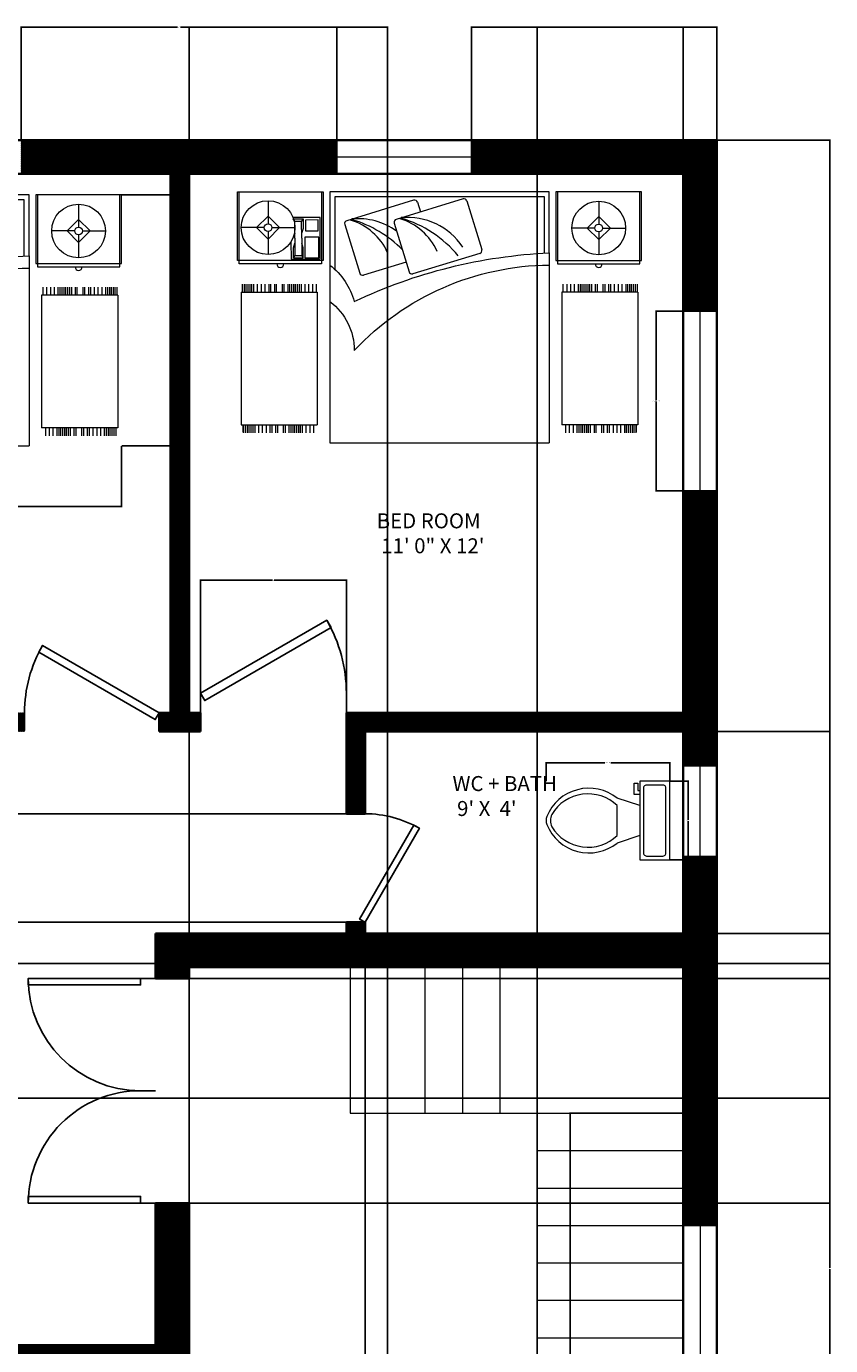
# Model space of a CAD drawing. Units: inches. Extents: x -24 to 516, y -23 to 640.
# Tile 5 of 5: x 302 to 516, y 288 to 640. Entities that reach past the tile are written whole.
import ezdxf

# ---------------------------------------------------------------- set-up
doc = ezdxf.new("R2010")
doc.units = ezdxf.units.IN
doc.header["$MEASUREMENT"] = 0
for name, color, linetype, lineweight in [('A-ANNO-DIMS', 2, 'Continuous', 18), ('A-AREA-IDEN', 7, 'Continuous', 18), ('A-FLOR-STRS', 7, 'Continuous', 18), ('A-WALL', 7, 'Continuous', 35), ('bathroom', 90, 'Continuous', 18), ('bedroom', 120, 'Continuous', 18), ('doors', 40, 'Continuous', 25), ('window', 30, 'Continuous', 18)]:
    doc.layers.add(name, color=color, linetype=linetype, lineweight=lineweight)
doc.layers.add('A-WALL-PATT', color=198, linetype='Continuous', lineweight=13, true_color=0x2e0f2e)
doc.styles.get("Standard").update_dxf_attribs({"font": 'arial.ttf'})
doc.dimstyles.get("Standard").update_dxf_attribs({"dimtxt": 0.18, "dimasz": 0.18, "dimexe": 0.18, "dimexo": 0.0625, "dimgap": 0.09, "dimtad": 0, "dimtih": 1, "dimtoh": 1, "dimdec": 4, "dimzin": 0, "dimdsep": 46, "dimtxsty": 'Standard', "dimcen": 0.09, "dimadec": 0, "dimazin": 0, "dimtfac": 1, "dimtdec": 4, "dimtofl": 0, "dimtmove": 0, "dimatfit": 3, "dimfxl": 1, "dimtolj": 1, "dimtzin": 0, "dimarcsym": 0})
pattern_1 = [(45, (-12045.43418, -42625.98622), (-0.08838834765, 0.08838834765), [])]

# ---------------------------------------------------------------- blocks, each defined once
blk = doc.blocks.new('*U6')
for p, q in [((0, 0), (0, -100)), ((750, 0), (750, -100))]:
    blk.add_line(p, q)
blk.add_lwpolyline([(0, 0), (649.5, 375), (671.4, 337.1), (21.9, -37.9)], close=True)
blk.add_arc((0, 0), 750, 0, 30)
blk = doc.blocks.new('*U7')
for p, q in [((0, 0), (0, 100)), ((750, 0), (750, 100))]:
    blk.add_line(p, q)
blk.add_lwpolyline([(0, 0), (649.5, -375), (671.4, -337.1), (21.9, 37.9)], close=True)
blk.add_arc((0, 0), 750, 330, 0)
blk = doc.blocks.new('*U9')
for p, q in [((0, 0), (0, -100)), ((750, 0), (750, -100))]:
    blk.add_line(p, q)
blk.add_lwpolyline([(0, 0), (0, 750), (43.75, 750), (43.75, 0)], close=True)
blk.add_arc((0, 0), 750, 0, 90)
blk = doc.blocks.new('3')
for p, q in [((185.866, 224.677), (185.866, 225.236)), ((185.866, 225.236), (186.566, 225.236)), ((185.88, 224.649), (185.88, 225.236)), ((186.552, 225.236), (186.552, 224.649)), ((186.566, 225.236), (186.566, 224.677)), ((186.62, 225.236), (186.62, 224.64)), ((188.409, 225.236), (186.62, 225.236)), ((188.409, 224.739), (188.409, 225.236)), ((188.463, 225.236), (188.463, 224.677)), ((189.162, 225.236), (188.463, 225.236)), ((188.477, 225.236), (188.477, 224.649)), ((189.148, 224.649), (189.148, 225.236)), ((189.162, 224.677), (189.162, 225.236)), ((186.116, 225.164), (186.116, 224.976)), ((187.303, 225.168), (186.758, 225.001)), ((187.706, 225.179), (187.161, 225.012)), ((187.334, 225.152), (187.359, 225.073)), ((187.737, 225.163), (187.858, 224.766)), ((188.812, 225.162), (188.812, 224.974)), ((186.022, 224.945), (186.116, 225.039)), ((186.116, 225.039), (186.21, 224.945)), ((186.54, 225.027), (186.319, 225.027)), ((186.321, 225.017), (186.401, 225.017)), ((186.401, 225.017), (186.389, 224.997)), ((186.401, 225.017), (186.401, 224.938)), ((186.541, 224.69), (186.54, 225.027)), ((188.812, 225.036), (188.718, 224.942)), ((188.907, 224.942), (188.812, 225.036)), ((186.084, 224.945), (185.896, 224.945)), ((186.116, 224.851), (186.022, 224.945)), ((186.21, 224.945), (186.116, 224.851)), ((186.116, 224.914), (186.116, 224.726)), ((186.147, 224.945), (186.335, 224.945)), ((186.333, 224.997), (186.321, 225.017)), ((186.334, 224.858), (186.333, 224.997)), ((186.333, 224.997), (186.389, 224.997)), ((186.39, 224.858), (186.389, 224.997)), ((186.401, 224.938), (186.389, 224.898)), ((186.742, 224.97), (186.863, 224.573)), ((187.144, 224.981), (187.266, 224.584)), ((188.781, 224.942), (188.593, 224.942)), ((188.718, 224.942), (188.812, 224.848)), ((188.812, 224.848), (188.907, 224.942)), ((188.812, 224.911), (188.812, 224.723)), ((188.844, 224.942), (189.032, 224.942)), ((186.302, 224.83), (186.303, 224.689)), ((186.322, 224.779), (186.334, 224.818)), ((186.331, 224.905), (186.334, 224.898)), ((186.334, 224.858), (186.334, 224.719)), ((186.39, 224.858), (186.39, 224.719)), ((186.402, 224.779), (186.39, 224.819)), ((186.323, 224.699), (186.322, 224.779)), ((186.334, 224.719), (186.323, 224.699)), ((186.323, 224.699), (186.402, 224.7)), ((186.334, 224.719), (186.39, 224.719)), ((186.402, 224.7), (186.39, 224.719)), ((186.402, 224.7), (186.402, 224.779)), ((187.842, 224.735), (187.297, 224.568)), ((188.409, 224.739), (188.409, 223.191)), ((186.566, 224.677), (185.866, 224.677)), ((186.552, 224.649), (185.88, 224.649)), ((186.303, 224.689), (186.541, 224.69)), ((186.62, 224.64), (186.62, 223.191)), ((187.242, 224.663), (186.894, 224.557)), ((188.463, 224.677), (189.162, 224.677)), ((188.477, 224.649), (189.148, 224.649)), ((185.904, 224.485, -0.909), (185.904, 224.42, -0.909)), ((185.92, 224.485, -0.909), (185.92, 224.42, -0.909)), ((185.92, 224.485, -0.909), (185.92, 224.42, -0.909)), ((185.935, 224.485, -0.909), (185.935, 224.42, -0.909)), ((185.951, 224.485, -0.909), (185.951, 224.42, -0.909)), ((185.966, 224.485, -0.909), (185.966, 224.42, -0.909)), ((185.982, 224.485, -0.909), (185.982, 224.42, -0.909)), ((185.997, 224.485, -0.909), (185.997, 224.42, -0.909)), ((186.028, 224.485, -0.909), (186.028, 224.42, -0.909)), ((186.059, 224.485, -0.909), (186.059, 224.42, -0.909)), ((186.09, 224.485, -0.909), (186.09, 224.42, -0.909)), ((186.09, 224.485, -0.909), (186.09, 224.42, -0.909)), ((186.121, 224.485, -0.909), (186.121, 224.42, -0.909)), ((186.137, 224.485, -0.909), (186.137, 224.42, -0.909)), ((186.168, 224.485, -0.909), (186.168, 224.42, -0.909)), ((186.183, 224.485, -0.909), (186.183, 224.42, -0.909)), ((186.23, 224.485, -0.909), (186.23, 224.42, -0.909)), ((186.245, 224.485, -0.909), (186.245, 224.42, -0.909)), ((186.276, 224.485, -0.909), (186.276, 224.42, -0.909)), ((186.292, 224.485, -0.909), (186.292, 224.42, -0.909)), ((186.307, 224.485, -0.909), (186.307, 224.42, -0.909)), ((186.323, 224.485, -0.909), (186.323, 224.42, -0.909)), ((186.338, 224.485, -0.909), (186.338, 224.42, -0.909)), ((186.354, 224.485, -0.909), (186.354, 224.42, -0.909)), ((186.369, 224.485, -0.909), (186.369, 224.42, -0.909)), ((186.385, 224.485, -0.909), (186.385, 224.42, -0.909)), ((186.416, 224.485, -0.909), (186.416, 224.42, -0.909)), ((186.447, 224.485, -0.909), (186.447, 224.42, -0.909)), ((186.478, 224.485, -0.909), (186.478, 224.42, -0.909)), ((186.509, 224.485, -0.909), (186.509, 224.42, -0.909)), ((188.52, 224.485, -0.909), (188.52, 224.42, -0.909)), ((188.551, 224.485, -0.909), (188.551, 224.42, -0.909)), ((188.582, 224.485, -0.909), (188.582, 224.42, -0.909)), ((188.613, 224.485, -0.909), (188.613, 224.42, -0.909)), ((188.644, 224.485, -0.909), (188.644, 224.42, -0.909)), ((188.66, 224.485, -0.909), (188.66, 224.42, -0.909)), ((188.675, 224.485, -0.909), (188.675, 224.42, -0.909)), ((188.691, 224.485, -0.909), (188.691, 224.42, -0.909)), ((188.706, 224.485, -0.909), (188.706, 224.42, -0.909)), ((188.722, 224.485, -0.909), (188.722, 224.42, -0.909)), ((188.737, 224.485, -0.909), (188.737, 224.42, -0.909)), ((188.753, 224.485, -0.909), (188.753, 224.42, -0.909)), ((188.784, 224.485, -0.909), (188.784, 224.42, -0.909)), ((188.799, 224.485, -0.909), (188.799, 224.42, -0.909)), ((188.846, 224.485, -0.909), (188.846, 224.42, -0.909)), ((188.861, 224.485, -0.909), (188.861, 224.42, -0.909)), ((188.892, 224.485, -0.909), (188.892, 224.42, -0.909)), ((188.908, 224.485, -0.909), (188.908, 224.42, -0.909)), ((188.939, 224.485, -0.909), (188.939, 224.42, -0.909)), ((188.939, 224.485, -0.909), (188.939, 224.42, -0.909)), ((188.97, 224.485, -0.909), (188.97, 224.42, -0.909)), ((189.001, 224.485, -0.909), (189.001, 224.42, -0.909)), ((189.032, 224.485, -0.909), (189.032, 224.42, -0.909)), ((189.047, 224.485, -0.909), (189.047, 224.42, -0.909)), ((189.063, 224.485, -0.909), (189.063, 224.42, -0.909)), ((189.078, 224.485, -0.909), (189.078, 224.42, -0.909)), ((189.094, 224.485, -0.909), (189.094, 224.42, -0.909)), ((189.109, 224.485, -0.909), (189.109, 224.42, -0.909)), ((189.109, 224.485, -0.909), (189.109, 224.42, -0.909)), ((189.125, 224.485, -0.909), (189.125, 224.42, -0.909)), ((185.897, 224.42, -0.909), (185.897, 223.338, -0.909)), ((185.897, 224.42, -0.909), (186.517, 224.42, -0.909)), ((186.517, 224.42, -0.909), (186.517, 223.338, -0.909)), ((189.131, 224.42, -0.909), (188.511, 224.42, -0.909)), ((188.511, 224.42, -0.909), (188.511, 223.338, -0.909)), ((189.131, 224.42, -0.909), (189.131, 223.338, -0.909)), ((185.897, 223.338, -0.909), (186.517, 223.338, -0.909)), ((185.911, 223.338, -0.909), (185.911, 223.279, -0.909)), ((185.911, 223.338, -0.909), (185.911, 223.279, -0.909)), ((185.911, 223.338, -0.909), (185.911, 223.279, -0.909)), ((185.914, 223.338, -0.909), (185.914, 223.273, -0.909)), ((185.929, 223.338, -0.909), (185.929, 223.273, -0.909)), ((185.929, 223.338, -0.909), (185.929, 223.273, -0.909)), ((185.945, 223.338, -0.909), (185.945, 223.273, -0.909)), ((185.96, 223.338, -0.909), (185.96, 223.273, -0.909)), ((185.976, 223.338, -0.909), (185.976, 223.273, -0.909)), ((185.991, 223.338, -0.909), (185.991, 223.273, -0.909)), ((186.007, 223.338, -0.909), (186.007, 223.273, -0.909)), ((186.038, 223.338, -0.909), (186.038, 223.273, -0.909)), ((186.069, 223.338, -0.909), (186.069, 223.273, -0.909)), ((186.1, 223.338, -0.909), (186.1, 223.273, -0.909)), ((186.1, 223.338, -0.909), (186.1, 223.273, -0.909)), ((186.131, 223.338, -0.909), (186.131, 223.273, -0.909)), ((186.146, 223.338, -0.909), (186.146, 223.273, -0.909)), ((186.177, 223.338, -0.909), (186.177, 223.273, -0.909)), ((186.193, 223.338, -0.909), (186.193, 223.273, -0.909)), ((186.239, 223.338, -0.909), (186.239, 223.273, -0.909)), ((186.255, 223.338, -0.909), (186.255, 223.273, -0.909)), ((186.286, 223.338, -0.909), (186.286, 223.273, -0.909)), ((186.301, 223.338, -0.909), (186.301, 223.273, -0.909)), ((186.317, 223.338, -0.909), (186.317, 223.273, -0.909)), ((186.332, 223.338, -0.909), (186.332, 223.273, -0.909)), ((186.348, 223.338, -0.909), (186.348, 223.273, -0.909)), ((186.363, 223.338, -0.909), (186.363, 223.273, -0.909)), ((186.379, 223.338, -0.909), (186.379, 223.273, -0.909)), ((186.394, 223.338, -0.909), (186.394, 223.273, -0.909)), ((186.425, 223.338, -0.909), (186.425, 223.273, -0.909)), ((186.456, 223.338, -0.909), (186.456, 223.273, -0.909)), ((186.487, 223.338, -0.909), (186.487, 223.273, -0.909)), ((189.131, 223.338, -0.909), (188.511, 223.338, -0.909)), ((188.541, 223.338, -0.909), (188.541, 223.273, -0.909)), ((188.572, 223.338, -0.909), (188.572, 223.273, -0.909)), ((188.603, 223.338, -0.909), (188.603, 223.273, -0.909)), ((188.634, 223.338, -0.909), (188.634, 223.273, -0.909)), ((188.65, 223.338, -0.909), (188.65, 223.273, -0.909)), ((188.665, 223.338, -0.909), (188.665, 223.273, -0.909)), ((188.681, 223.338, -0.909), (188.681, 223.273, -0.909)), ((188.696, 223.338, -0.909), (188.696, 223.273, -0.909)), ((188.712, 223.338, -0.909), (188.712, 223.273, -0.909)), ((188.727, 223.338, -0.909), (188.727, 223.273, -0.909)), ((188.743, 223.338, -0.909), (188.743, 223.273, -0.909)), ((188.774, 223.338, -0.909), (188.774, 223.273, -0.909)), ((188.789, 223.338, -0.909), (188.789, 223.273, -0.909)), ((188.836, 223.338, -0.909), (188.836, 223.273, -0.909)), ((188.851, 223.338, -0.909), (188.851, 223.273, -0.909)), ((188.882, 223.338, -0.909), (188.882, 223.273, -0.909)), ((188.898, 223.338, -0.909), (188.898, 223.273, -0.909)), ((188.929, 223.338, -0.909), (188.929, 223.273, -0.909)), ((188.929, 223.338, -0.909), (188.929, 223.273, -0.909)), ((188.96, 223.338, -0.909), (188.96, 223.273, -0.909)), ((188.991, 223.338, -0.909), (188.991, 223.273, -0.909)), ((189.022, 223.338, -0.909), (189.022, 223.273, -0.909)), ((189.037, 223.338, -0.909), (189.037, 223.273, -0.909)), ((189.053, 223.338, -0.909), (189.053, 223.273, -0.909)), ((189.068, 223.338, -0.909), (189.068, 223.273, -0.909)), ((189.084, 223.338, -0.909), (189.084, 223.273, -0.909)), ((189.099, 223.338, -0.909), (189.099, 223.273, -0.909)), ((189.099, 223.338, -0.909), (189.099, 223.273, -0.909)), ((189.115, 223.338, -0.909), (189.115, 223.273, -0.909)), ((189.117, 223.338, -0.909), (189.117, 223.279, -0.909)), ((189.117, 223.338, -0.909), (189.117, 223.279, -0.909)), ((189.117, 223.338, -0.909), (189.117, 223.279, -0.909)), ((186.62, 223.191), (188.409, 223.191))]:
    blk.add_line(p, q)
blk.add_lwpolyline([(188.369, 224.737), (188.369, 225.197), (186.66, 225.197), (186.66, 224.606)])
for points in [[(186.422, 225.007), (186.422, 224.92), (186.525, 224.92), (186.525, 225.008)], [(186.415, 224.866), (186.416, 224.7), (186.531, 224.7), (186.53, 224.867)]]:
    blk.add_lwpolyline(points, close=True)
for points in [[(186.62, 224.64, -0.162278), (186.819, 224.342, -0.100664), (188.409, 224.739, -0.100664)], [(186.62, 224.342, -0.236068), (186.819, 223.944, -0.205258), (188.409, 224.64, -0.205258)]]:
    blk.add_lwpolyline(points, format="xyb")
for centre, radius in [((186.116, 224.945), 0.219), ((188.812, 224.942), 0.219), ((186.116, 224.945), 0.0313), ((188.812, 224.942), 0.0313)]:
    blk.add_circle(centre, radius)
for centre, radius, start, end in [((187.311, 225.145), 0.0248, 17.0142, 107.0142), ((187.713, 225.156), 0.0248, 17.0142, 107.0142), ((186.848, 224.471), 0.547, 54.6851, 95.1605), ((187.05, 224.552), 0.487, 24.2209, 73.0691), ((187.25, 224.482), 0.547, 33.7801, 95.1605), ((186.938, 224.116), 0.943, 39.4023, 73.7189), ((186.765, 224.978), 0.0248, 107.0142, 197.0142), ((186.647, 224.541), 0.487, 24.2209, 73.0691), ((186.536, 224.105), 0.943, 44.2727, 73.7189), ((187.168, 224.989), 0.0248, 107.0142, 197.0142), ((187.835, 224.758), 0.0248, 287.0142, 17.0142), ((186.216, 224.649), 0.028, 180, 0), ((188.812, 224.649), 0.028, 180, 0), ((186.887, 224.581), 0.0248, 197.0142, 287.0142), ((187.289, 224.592), 0.0248, 197.0142, 287.0142)]:
    blk.add_arc(centre, radius, start, end)
blk = doc.blocks.new('Toilet - top')
for p, q in [((9.5, -6), (9.5, -2)), ((-10, -8.5), (-8, -8.5)), ((-10, -9.5), (-10, -8.5)), ((-7, -9.5), (-10, -9.5)), ((-8, -8.5), (-8, -8)), ((-7, -8), (-7, -9.5)), ((-4, -8), (-6, -14)), ((4, -8), (6, -14)), ((4, -14), (-4, -14))]:
    blk.add_line(p, q)
blk.add_lwpolyline([(10.5, -8), (10.5, 0), (-10.5, 0), (-10.5, -8)], close=True)
for points in [[(-9.5, -2), (-9.5, -6)], [(8.5, -1), (-8.5, -1)], [(-8.5, -7), (8.5, -7)]]:
    blk.add_lwpolyline(points)
for centre, radius, start, end in [((-8.62, -1.88), 0.884, 81.8699, 188.1301), ((8.62, -1.88), 0.884, 351.8699, 98.1301), ((-8.62, -6.12), 0.884, 171.8699, 278.1301), ((8.62, -6.12), 0.884, 261.8699, 8.1301), ((3.52, -21.58), 12.17, 141.4691, 247.9714), ((4.2, -21.82), 11.33, 136.3677, 238.9468), ((-3.52, -21.58), 12.17, 292.0284, 38.5307), ((-4.2, -21.82), 11.33, 301.053, 43.6321), ((0, -27.88), 4, 245.7318, 294.2682), ((0, -29), 4, 254.8605, 285.1395)]:
    blk.add_arc(centre, radius, start, end)
blk = doc.blocks.new('WIN-36IN')
for p, q in [((0, 0), (0, 36)), ((0, 36), (9, 36)), ((4.5, 0), (4.5, 36)), ((9, 36), (9, 0)), ((9, 0), (0, 0)), ((9, 0), (4.5, 0))]:
    blk.add_line(p, q)
blk = doc.blocks.new('WIN-24IN')
for p, q in [((0, 0), (0, 24)), ((0, 24), (9, 24)), ((4.5, 0), (4.5, 24)), ((9, 24), (9, 0)), ((9, 0), (0, 0)), ((9, 0), (4.5, 0))]:
    blk.add_line(p, q)
blk = doc.blocks.new('WIN-48IN')
for p, q in [((0, 48), (9, 48)), ((0, 0), (0, 48)), ((4.5, 48), (4.5, 0)), ((9, 48), (9, 0)), ((9, 0), (0, 0))]:
    blk.add_line(p, q)
blk = doc.blocks.new('*D15')
at = {"layer": 'A-ANNO-DIMS', "color": 0, "lineweight": -2, "transparency": 16777216}
for p, q in [((219.01, 528.26), (219.01, 511.94)), ((327.01, 528.26), (327.01, 511.94)), ((219.19, 512.12), (271.63, 512.12)), ((326.83, 512.12), (274.4, 512.12))]:
    blk.add_line(p, q, dxfattribs=at)
at = {"layer": 'A-ANNO-DIMS', "color": 0, "transparency": 16777216}
for points in [[(219.19, 512.15), (219.19, 512.09), (219.01, 512.12)], [(326.83, 512.15), (326.83, 512.09), (327.01, 512.12)]]:
    blk.add_solid(points, dxfattribs=at)
at = {"layer": 'Defpoints', "color": 0, "transparency": 16777216}
for p in [(219.01, 528.32), (327.01, 528.32), (327.01, 512.12)]:
    blk.add_point(p, dxfattribs=at)
at = {"layer": 'A-ANNO-DIMS', "color": 0, "transparency": 16777216, "insert": (273.01, 512.12), "char_height": 0.18, "attachment_point": 5}
blk.add_mtext('\\A1;BED GROUP 108 TYP.', dxfattribs=at)
blk = doc.blocks.new('*D16')
at = {"layer": 'A-ANNO-DIMS', "color": 0, "lineweight": -2, "transparency": 16777216}
for p, q in [((327.08, 595.36), (343.39, 595.36)), ((343.21, 595.18), (343.21, 562.02)), ((343.21, 528.5), (343.21, 561.66)), ((327.08, 528.32), (343.39, 528.32))]:
    blk.add_line(p, q, dxfattribs=at)
at = {"layer": 'A-ANNO-DIMS', "color": 0, "transparency": 16777216}
for points in [[(343.18, 595.18), (343.24, 595.18), (343.21, 595.36)], [(343.18, 528.5), (343.24, 528.5), (343.21, 528.32)]]:
    blk.add_solid(points, dxfattribs=at)
at = {"layer": 'Defpoints', "color": 0, "transparency": 16777216}
for p in [(327.01, 595.36), (343.21, 595.36), (327.01, 528.32)]:
    blk.add_point(p, dxfattribs=at)
at = {"layer": 'A-ANNO-DIMS', "color": 0, "transparency": 16777216, "insert": (343.21, 561.84), "char_height": 0.18, "attachment_point": 5}
blk.add_mtext('\\A1;67 TYP.', dxfattribs=at)
blk = doc.blocks.new('*D17')
at = {"layer": 'A-ANNO-DIMS', "color": 0, "lineweight": -2, "transparency": 16777216}
for p, q in [((440.43, 438.76), (440.43, 443.83)), ((440.61, 443.65), (456.18, 443.65)), ((473.3, 443.65), (457.73, 443.65)), ((473.48, 438.76), (473.48, 443.83))]:
    blk.add_line(p, q, dxfattribs=at)
at = {"layer": 'A-ANNO-DIMS', "color": 0, "transparency": 16777216}
for points in [[(440.61, 443.68), (440.61, 443.62), (440.43, 443.65)], [(473.3, 443.68), (473.3, 443.62), (473.48, 443.65)]]:
    blk.add_solid(points, dxfattribs=at)
at = {"layer": 'Defpoints', "color": 0, "transparency": 16777216}
for p in [(473.48, 443.65), (440.43, 438.69), (473.48, 438.69)]:
    blk.add_point(p, dxfattribs=at)
at = {"layer": 'A-ANNO-DIMS', "color": 0, "transparency": 16777216, "insert": (456.96, 443.65), "char_height": 0.18, "attachment_point": 5}
blk.add_mtext('\\A1;WC 33 TYP.', dxfattribs=at)
blk = doc.blocks.new('*D18')
at = {"layer": 'A-ANNO-DIMS', "color": 0, "lineweight": -2, "transparency": 16777216}
for p, q in [((473.54, 438.69), (478.62, 438.69)), ((478.44, 438.51), (478.44, 428.38)), ((478.44, 417.87), (478.44, 428.01)), ((473.54, 417.69), (478.62, 417.69))]:
    blk.add_line(p, q, dxfattribs=at)
at = {"layer": 'A-ANNO-DIMS', "color": 0, "transparency": 16777216}
for points in [[(478.41, 438.51), (478.47, 438.51), (478.44, 438.69)], [(478.41, 417.87), (478.47, 417.87), (478.44, 417.69)]]:
    blk.add_solid(points, dxfattribs=at)
at = {"layer": 'Defpoints', "color": 0, "transparency": 16777216}
for p in [(473.48, 438.69), (473.48, 417.69), (478.44, 417.69)]:
    blk.add_point(p, dxfattribs=at)
at = {"layer": 'A-ANNO-DIMS', "color": 0, "transparency": 16777216, "insert": (478.44, 428.19), "char_height": 0.18, "attachment_point": 5}
blk.add_mtext('\\A1;21 TYP.', dxfattribs=at)
blk = doc.blocks.new('*D23')
at = {"layer": 'A-ANNO-DIMS', "color": 0, "lineweight": -2, "transparency": 16777216}
for p, q in [((477.03, 564.3), (469.71, 564.3)), ((469.89, 564.12), (469.89, 540.49)), ((469.89, 516.48), (469.89, 540.12)), ((477.03, 516.3), (469.71, 516.3))]:
    blk.add_line(p, q, dxfattribs=at)
at = {"layer": 'A-ANNO-DIMS', "color": 0, "transparency": 16777216}
for points in [[(469.86, 564.12), (469.92, 564.12), (469.89, 564.3)], [(469.86, 516.48), (469.92, 516.48), (469.89, 516.3)]]:
    blk.add_solid(points, dxfattribs=at)
at = {"layer": 'Defpoints', "color": 0, "transparency": 16777216}
for p in [(477.09, 564.3), (469.89, 516.3), (477.09, 516.3)]:
    blk.add_point(p, dxfattribs=at)
at = {"layer": 'A-ANNO-DIMS', "color": 0, "transparency": 16777216, "insert": (469.89, 540.3), "char_height": 0.18, "attachment_point": 5}
blk.add_mtext('\\A1;WINDOW 48 TYP.', dxfattribs=at)
blk = doc.blocks.new('*D24')
at = {"layer": 'A-ANNO-DIMS', "color": 0, "lineweight": -2, "transparency": 16777216}
for p, q in [((477.09, 564.36), (477.09, 571.68)), ((477.27, 571.5), (481.13, 571.5)), ((485.91, 571.5), (482.05, 571.5)), ((486.09, 564.36), (486.09, 571.68))]:
    blk.add_line(p, q, dxfattribs=at)
at = {"layer": 'A-ANNO-DIMS', "color": 0, "transparency": 16777216}
for points in [[(477.27, 571.53), (477.27, 571.47), (477.09, 571.5)], [(485.91, 571.53), (485.91, 571.47), (486.09, 571.5)]]:
    blk.add_solid(points, dxfattribs=at)
at = {"layer": 'Defpoints', "color": 0, "transparency": 16777216}
for p in [(477.09, 571.5), (477.09, 564.3), (486.09, 564.3)]:
    blk.add_point(p, dxfattribs=at)
at = {"layer": 'A-ANNO-DIMS', "color": 0, "transparency": 16777216, "insert": (481.59, 571.5), "char_height": 0.18, "attachment_point": 5}
blk.add_mtext('\\A1;9 TYP.', dxfattribs=at)
blk = doc.blocks.new('*D34')
at = {"layer": 'A-ANNO-DIMS', "color": 0, "lineweight": -2, "transparency": 16777216}
for p, q in [((486.15, 610.01), (516.45, 610.01)), ((516.27, 609.83), (516.27, 308.7)), ((516.27, 7.19), (516.27, 308.33)), ((486.15, 7.01), (516.45, 7.01))]:
    blk.add_line(p, q, dxfattribs=at)
at = {"layer": 'A-ANNO-DIMS', "color": 0, "transparency": 16777216}
for points in [[(516.24, 609.83), (516.3, 609.83), (516.27, 610.01)], [(516.24, 7.19), (516.3, 7.19), (516.27, 7.01)]]:
    blk.add_solid(points, dxfattribs=at)
at = {"layer": 'Defpoints', "color": 0, "transparency": 16777216}
for p in [(486.09, 610.01), (516.27, 610.01), (486.09, 7.01)]:
    blk.add_point(p, dxfattribs=at)
at = {"layer": 'A-ANNO-DIMS', "color": 0, "transparency": 16777216, "insert": (516.27, 308.51), "char_height": 0.18, "attachment_point": 5}
blk.add_mtext('\\A1;603', dxfattribs=at)
blk = doc.blocks.new('*D48')
at = {"layer": 'A-ANNO-DIMS', "color": 0, "lineweight": -2, "transparency": 16777216}
for p, q in [((99.15, 390.01), (516.45, 390.01)), ((516.27, 389.83), (516.27, 372.2)), ((516.27, 354.19), (516.27, 371.83)), ((99.15, 354.01), (516.45, 354.01))]:
    blk.add_line(p, q, dxfattribs=at)
at = {"layer": 'A-ANNO-DIMS', "color": 0, "transparency": 16777216}
for points in [[(516.24, 389.83), (516.3, 389.83), (516.27, 390.01)], [(516.24, 354.19), (516.3, 354.19), (516.27, 354.01)]]:
    blk.add_solid(points, dxfattribs=at)
at = {"layer": 'Defpoints', "color": 0, "transparency": 16777216}
for p in [(99.09, 390.01), (516.27, 390.01), (99.09, 354.01)]:
    blk.add_point(p, dxfattribs=at)
at = {"layer": 'A-ANNO-DIMS', "color": 0, "transparency": 16777216, "insert": (516.27, 372.01), "char_height": 0.18, "attachment_point": 5}
blk.add_mtext('\\A1;36', dxfattribs=at)
blk = doc.blocks.new('*D49')
at = {"layer": 'A-ANNO-DIMS', "color": 0, "lineweight": -2, "transparency": 16777216}
for p, q in [((345.09, 173.08), (345.09, 640.38)), ((345.27, 640.2), (371.37, 640.2)), ((397.91, 640.2), (371.81, 640.2)), ((398.09, 173.08), (398.09, 640.38))]:
    blk.add_line(p, q, dxfattribs=at)
at = {"layer": 'A-ANNO-DIMS', "color": 0, "transparency": 16777216}
for points in [[(345.27, 640.23), (345.27, 640.17), (345.09, 640.2)], [(397.91, 640.23), (397.91, 640.17), (398.09, 640.2)]]:
    blk.add_solid(points, dxfattribs=at)
at = {"layer": 'Defpoints', "color": 0, "transparency": 16777216}
for p in [(398.09, 640.2), (345.09, 173.01), (398.09, 173.01)]:
    blk.add_point(p, dxfattribs=at)
at = {"layer": 'A-ANNO-DIMS', "color": 0, "transparency": 16777216, "insert": (371.59, 640.2), "char_height": 0.18, "attachment_point": 5}
blk.add_mtext('\\A1;53', dxfattribs=at)
blk = doc.blocks.new('*D50')
at = {"layer": 'A-ANNO-DIMS', "color": 0, "lineweight": -2, "transparency": 16777216}
for p, q in [((336.15, 386.01), (516.45, 386.01)), ((516.27, 385.83), (516.27, 356.2)), ((516.27, 326.19), (516.27, 355.83)), ((336.15, 326.01), (516.45, 326.01))]:
    blk.add_line(p, q, dxfattribs=at)
at = {"layer": 'A-ANNO-DIMS', "color": 0, "transparency": 16777216}
for points in [[(516.24, 385.83), (516.3, 385.83), (516.27, 386.01)], [(516.24, 326.19), (516.3, 326.19), (516.27, 326.01)]]:
    blk.add_solid(points, dxfattribs=at)
at = {"layer": 'Defpoints', "color": 0, "transparency": 16777216}
for p in [(336.09, 386.01), (516.27, 386.01), (336.09, 326.01)]:
    blk.add_point(p, dxfattribs=at)
at = {"layer": 'A-ANNO-DIMS', "color": 0, "transparency": 16777216, "insert": (516.27, 356.01), "char_height": 0.18, "attachment_point": 5}
blk.add_mtext('\\A1;60', dxfattribs=at)
blk = doc.blocks.new('*D51')
at = {"layer": 'A-ANNO-DIMS', "color": 0, "lineweight": -2, "transparency": 16777216}
for p, q in [((438.09, 221.08), (438.09, 640.38)), ((438.27, 640.2), (457.37, 640.2)), ((476.91, 640.2), (457.81, 640.2)), ((477.09, 221.08), (477.09, 640.38))]:
    blk.add_line(p, q, dxfattribs=at)
at = {"layer": 'A-ANNO-DIMS', "color": 0, "transparency": 16777216}
for points in [[(438.27, 640.23), (438.27, 640.17), (438.09, 640.2)], [(476.91, 640.23), (476.91, 640.17), (477.09, 640.2)]]:
    blk.add_solid(points, dxfattribs=at)
at = {"layer": 'Defpoints', "color": 0, "transparency": 16777216}
for p in [(477.09, 640.2), (438.09, 221.01), (477.09, 221.01)]:
    blk.add_point(p, dxfattribs=at)
at = {"layer": 'A-ANNO-DIMS', "color": 0, "transparency": 16777216, "insert": (457.59, 640.2), "char_height": 0.18, "attachment_point": 5}
blk.add_mtext('\\A1;39', dxfattribs=at)
blk = doc.blocks.new('*D52')
at = {"layer": 'A-ANNO-DIMS', "color": 0, "lineweight": -2, "transparency": 16777216}
for p, q in [((392.03, 430.01), (-24.28, 430.01)), ((-24.1, 429.83), (-24.1, 415.7)), ((-24.1, 401.19), (-24.1, 415.33)), ((392.03, 401.01), (-24.28, 401.01))]:
    blk.add_line(p, q, dxfattribs=at)
at = {"layer": 'A-ANNO-DIMS', "color": 0, "transparency": 16777216}
for points in [[(-24.13, 429.83), (-24.07, 429.83), (-24.1, 430.01)], [(-24.13, 401.19), (-24.07, 401.19), (-24.1, 401.01)]]:
    blk.add_solid(points, dxfattribs=at)
at = {"layer": 'Defpoints', "color": 0, "transparency": 16777216}
for p in [(-24.1, 430.01), (392.09, 430.01), (392.09, 401.01)]:
    blk.add_point(p, dxfattribs=at)
at = {"layer": 'A-ANNO-DIMS', "color": 0, "transparency": 16777216, "insert": (-24.1, 415.51), "char_height": 0.18, "attachment_point": 5}
blk.add_mtext('\\A1;29', dxfattribs=at)
blk = doc.blocks.new('*D53')
at = {"layer": 'A-ANNO-DIMS', "color": 0, "lineweight": -2, "transparency": 16777216}
for p, q in [((477.15, 452.01), (516.45, 452.01)), ((516.27, 451.83), (516.27, 425.19)), ((516.27, 398.19), (516.27, 424.83)), ((477.15, 398.01), (516.45, 398.01))]:
    blk.add_line(p, q, dxfattribs=at)
at = {"layer": 'A-ANNO-DIMS', "color": 0, "transparency": 16777216}
for points in [[(516.24, 451.83), (516.3, 451.83), (516.27, 452.01)], [(516.24, 398.19), (516.3, 398.19), (516.27, 398.01)]]:
    blk.add_solid(points, dxfattribs=at)
at = {"layer": 'Defpoints', "color": 0, "transparency": 16777216}
for p in [(477.09, 452.01), (516.27, 452.01), (477.09, 398.01)]:
    blk.add_point(p, dxfattribs=at)
at = {"layer": 'A-ANNO-DIMS', "color": 0, "transparency": 16777216, "insert": (516.27, 425.01), "char_height": 0.18, "attachment_point": 5}
blk.add_mtext('\\A1;54', dxfattribs=at)
blk = doc.blocks.new('*D54')
at = {"layer": 'A-ANNO-DIMS', "color": 0, "lineweight": -2, "transparency": 16777216}
for p, q in [((392.09, 397.95), (392.09, -23.35)), ((477.09, 397.95), (477.09, -23.35)), ((392.27, -23.17), (434.37, -23.17)), ((476.91, -23.17), (434.81, -23.17))]:
    blk.add_line(p, q, dxfattribs=at)
at = {"layer": 'A-ANNO-DIMS', "color": 0, "transparency": 16777216}
for points in [[(392.27, -23.14), (392.27, -23.2), (392.09, -23.17)], [(476.91, -23.14), (476.91, -23.2), (477.09, -23.17)]]:
    blk.add_solid(points, dxfattribs=at)
at = {"layer": 'Defpoints', "color": 0, "transparency": 16777216}
for p in [(392.09, 398.01), (477.09, 398.01), (477.09, -23.17)]:
    blk.add_point(p, dxfattribs=at)
at = {"layer": 'A-ANNO-DIMS', "color": 0, "transparency": 16777216, "insert": (434.59, -23.17), "char_height": 0.18, "attachment_point": 5}
blk.add_mtext('\\A1;85', dxfattribs=at)
blk = doc.blocks.new('*D59')
at = {"layer": 'A-ANNO-DIMS', "color": 0, "lineweight": -2, "transparency": 16777216}
for p, q in [((477.03, 350.01), (446.72, 350.01)), ((446.9, 349.83), (446.9, 285.7)), ((446.9, 221.19), (446.9, 285.33)), ((477.03, 221.01), (446.72, 221.01))]:
    blk.add_line(p, q, dxfattribs=at)
at = {"layer": 'A-ANNO-DIMS', "color": 0, "transparency": 16777216}
for points in [[(446.87, 349.83), (446.93, 349.83), (446.9, 350.01)], [(446.87, 221.19), (446.93, 221.19), (446.9, 221.01)]]:
    blk.add_solid(points, dxfattribs=at)
at = {"layer": 'Defpoints', "color": 0, "transparency": 16777216}
for p in [(446.9, 350.01), (477.09, 350.01), (477.09, 221.01)]:
    blk.add_point(p, dxfattribs=at)
at = {"layer": 'A-ANNO-DIMS', "color": 0, "transparency": 16777216, "insert": (446.9, 285.51), "char_height": 0.18, "attachment_point": 5}
blk.add_mtext('\\A1;129', dxfattribs=at)
blk = doc.blocks.new('*D60')
at = {"layer": 'A-ANNO-DIMS', "color": 0, "lineweight": -2, "transparency": 16777216}
for p, q in [((348.09, 462.28), (348.09, 492.58)), ((348.27, 492.4), (367.37, 492.4)), ((386.91, 492.4), (367.81, 492.4)), ((387.09, 462.28), (387.09, 492.58))]:
    blk.add_line(p, q, dxfattribs=at)
at = {"layer": 'A-ANNO-DIMS', "color": 0, "transparency": 16777216}
for points in [[(348.27, 492.43), (348.27, 492.37), (348.09, 492.4)], [(386.91, 492.43), (386.91, 492.37), (387.09, 492.4)]]:
    blk.add_solid(points, dxfattribs=at)
at = {"layer": 'Defpoints', "color": 0, "transparency": 16777216}
for p in [(387.09, 492.4), (348.09, 462.21), (387.09, 462.21)]:
    blk.add_point(p, dxfattribs=at)
at = {"layer": 'A-ANNO-DIMS', "color": 0, "transparency": 16777216, "insert": (367.59, 492.4), "char_height": 0.18, "attachment_point": 5}
blk.add_mtext('\\A1;39', dxfattribs=at)
blk = doc.blocks.new('*D64')
at = {"layer": 'A-ANNO-DIMS', "color": 0, "lineweight": -2, "transparency": 16777216}
for p, q in [((300.21, 610.08), (300.21, 640.38)), ((300.39, 640.2), (341.99, 640.2)), ((384.38, 640.2), (342.78, 640.2)), ((384.56, 610.08), (384.56, 640.38))]:
    blk.add_line(p, q, dxfattribs=at)
at = {"layer": 'A-ANNO-DIMS', "color": 0, "transparency": 16777216}
for points in [[(300.39, 640.23), (300.39, 640.17), (300.21, 640.2)], [(384.38, 640.23), (384.38, 640.17), (384.56, 640.2)]]:
    blk.add_solid(points, dxfattribs=at)
at = {"layer": 'Defpoints', "color": 0, "transparency": 16777216}
for p in [(384.56, 640.2), (300.21, 610.01), (384.56, 610.01)]:
    blk.add_point(p, dxfattribs=at)
at = {"layer": 'A-ANNO-DIMS', "color": 0, "transparency": 16777216, "insert": (342.38, 640.2), "char_height": 0.18, "attachment_point": 5}
blk.add_mtext('\\A1;84.35', dxfattribs=at)
blk = doc.blocks.new('*D65')
at = {"layer": 'A-ANNO-DIMS', "color": 0, "lineweight": -2, "transparency": 16777216}
for p, q in [((420.56, 610.08), (420.56, 640.38)), ((420.74, 640.2), (452.93, 640.2)), ((485.91, 640.2), (453.72, 640.2)), ((486.09, 610.08), (486.09, 640.38))]:
    blk.add_line(p, q, dxfattribs=at)
at = {"layer": 'A-ANNO-DIMS', "color": 0, "transparency": 16777216}
for points in [[(420.74, 640.23), (420.74, 640.17), (420.56, 640.2)], [(485.91, 640.23), (485.91, 640.17), (486.09, 640.2)]]:
    blk.add_solid(points, dxfattribs=at)
at = {"layer": 'Defpoints', "color": 0, "transparency": 16777216}
for p in [(486.09, 640.2), (420.56, 610.01), (486.09, 610.01)]:
    blk.add_point(p, dxfattribs=at)
at = {"layer": 'A-ANNO-DIMS', "color": 0, "transparency": 16777216, "insert": (453.32, 640.2), "char_height": 0.18, "attachment_point": 5}
blk.add_mtext('\\A1;65.53', dxfattribs=at)

msp = doc.modelspace()

# ---------------------------------------------------------------- hatches: boundary and pattern name
at = {"layer": 'A-WALL-PATT'}
h = msp.add_hatch(dxfattribs=at)
h.set_pattern_fill('ANSI31', color=256)
h.set_pattern_definition(pattern_1)
h.paths.add_polyline_path([(15.088, 601.013), (52.998, 601.013), (52.998, 610.013), (6.088, 610.013), (6.088, 554.753), (15.088, 554.753)])
h.paths.add_polyline_path([(171.065, 610.013), (88.998, 610.013), (88.998, 601.013), (150.088, 601.013), (150.088, 457.013), (147.088, 457.013), (147.088, 452.013), (155.088, 452.013), (155.088, 488.013), (203.088, 488.013), (203.088, 452.013), (301.088, 452.013), (301.088, 457.013), (208.088, 457.013), (208.088, 496.013), (203.088, 496.013), (203.088, 493.013), (155.088, 493.013), (155.088, 601.013), (171.065, 601.013)])
h.paths.add_polyline_path([(264.208, 610.013), (195.065, 610.013), (195.065, 601.013), (203.088, 601.013), (203.088, 525.013), (208.088, 525.013), (208.088, 601.013), (264.208, 601.013)], flags=17)
h.paths.add_polyline_path([(384.556, 610.013), (300.208, 610.013), (300.208, 601.013), (340.088, 601.013), (340.088, 457.013), (337.088, 456.991), (337.088, 452.013), (340.088, 452.013), (348.088, 452.013), (348.088, 457.013), (345.088, 457.013), (345.088, 601.013), (384.556, 601.013)])
h.paths.add_polyline_path([(486.088, 610.013), (420.556, 610.013), (420.556, 601.013), (477.088, 601.013), (477.088, 564.302), (486.088, 564.302)])
h.paths.add_polyline_path([(486.088, 516.302), (477.088, 516.302), (477.088, 457.013), (387.088, 457.013), (387.088, 430.013), (392.088, 430.013), (392.088, 452.013), (477.088, 452.013), (477.088, 442.706), (486.088, 442.706)])
h.paths.add_polyline_path([(486.088, 418.706), (477.088, 418.706), (477.088, 398.013), (392.088, 398.013), (392.088, 401.013), (388.222, 401.013), (387.088, 401.013), (387.088, 398.013), (336.088, 398.013), (336.088, 386.013), (345.088, 386.013), (345.088, 389.013), (477.088, 389.013), (477.088, 320.013), (486.088, 320.013)])
h.paths.add_polyline_path([(486.088, 272.013), (477.088, 272.013), (477.088, 182.013), (398.088, 182.013), (398.088, 173.013), (486.088, 173.013)])
h = msp.add_hatch(dxfattribs=at)
h.set_pattern_fill('ANSI31', color=256)
h.set_pattern_definition(pattern_1)
h.paths.add_polyline_path([(161.63, 139.013), (155.088, 139.013), (155.088, 283.013), (203.088, 283.013), (203.088, 171.013), (208.088, 171.013), (208.088, 283.013), (211.088, 283.013), (211.088, 288.013), (208.088, 288.013), (147.088, 288.013), (147.088, 283.013), (150.088, 283.013), (150.088, 139.013), (87.664, 139.013), (87.664, 134.513), (87.664, 130.013), (161.63, 130.013)])
h.paths.add_polyline_path([(256.352, 139.013), (208.088, 139.013), (208.088, 142.013), (203.088, 142.013), (203.088, 139.013), (185.63, 139.013), (185.63, 130.013), (256.352, 130.013)])
h.paths.add_polyline_path([(345.088, 326.013), (336.088, 326.013), (336.088, 288.013), (247.088, 288.013), (247.088, 283.013), (340.088, 283.013), (340.088, 139.013), (292.352, 139.013), (292.352, 134.513), (292.352, 130.013), (345.088, 130.013)])
h.paths.add_polyline_path([(51.664, 139.013), (15.088, 139.013), (15.088, 195.946), (10.588, 195.946), (6.088, 195.946), (6.088, 130.013), (51.664, 130.013)])
h.paths.add_polyline_path([(15.088, 283.013), (111.088, 283.013), (111.088, 288.013), (104.088, 288.013), (104.088, 354.013), (99.088, 354.013), (99.088, 288.013), (15.088, 288.013), (15.088, 324.046), (10.588, 324.046), (6.088, 324.046), (6.088, 231.946), (15.088, 231.946)])
h.paths.add_polyline_path([(15.088, 398.013), (99.088, 398.013), (99.088, 390.013), (104.088, 390.013), (104.088, 393.013), (104.088, 407.013), (99.088, 407.013), (99.088, 404.013), (15.088, 404.013), (15.088, 416.474), (10.588, 416.474), (6.088, 416.474), (6.088, 360.046), (15.088, 360.046)])
h.paths.add_polyline_path([(15.088, 518.753), (10.588, 518.753), (6.088, 518.753), (6.088, 440.474), (15.088, 440.474), (15.088, 452.013), (99.088, 452.013), (99.088, 436.013), (104.088, 436.013), (104.088, 452.013), (111.088, 452.013), (111.088, 457.013), (15.088, 457.013)])

# ---------------------------------------------------------------- linework, layer by layer
at = {"layer": 'A-FLOR-STRS'}
for p, q in [((388.088, 389.013), (388.088, 350.013)), ((398.088, 389.013), (398.088, 350.013)), ((408.088, 389.013), (408.088, 350.013)), ((418.088, 389.013), (418.088, 350.013)), ((428.088, 389.013), (428.088, 350.013)), ((438.088, 320.013), (438.088, 389.013)), ((438.088, 389.013), (438.088, 221.013)), ((388.088, 350.013), (477.088, 350.013)), ((438.088, 340.013), (477.088, 340.013)), ((438.088, 330.013), (477.088, 330.013)), ((438.088, 320.013), (477.088, 320.013)), ((438.088, 310.013), (477.088, 310.013)), ((438.088, 300.013), (477.088, 300.013)), ((438.088, 290.013), (477.088, 290.013))]:
    msp.add_line(p, q, dxfattribs=at)
at = {"layer": 'A-WALL'}
for p, q in [((208.088, 601.013), (340.088, 601.013)), ((340.088, 457.013), (340.088, 601.013)), ((345.088, 601.013), (477.088, 601.013)), ((345.088, 457.013), (345.088, 601.013)), ((477.088, 601.013), (477.088, 457.013)), ((340.088, 457.013), (337.088, 456.991)), ((337.088, 456.991), (337.088, 452.013)), ((345.088, 457.013), (348.088, 457.013)), ((345.088, 457.013), (348.088, 457.013)), ((348.088, 457.013), (348.088, 452.013)), ((387.088, 457.013), (477.088, 457.013)), ((387.088, 457.013), (387.088, 430.013)), ((337.088, 452.013), (348.088, 452.013)), ((337.088, 452.013), (340.088, 452.013)), ((392.088, 452.013), (477.088, 452.013)), ((392.088, 452.013), (392.088, 430.013)), ((477.088, 452.013), (477.088, 398.013)), ((392.088, 430.013), (387.088, 430.013)), ((387.088, 401.013), (387.088, 398.013)), ((392.088, 401.013), (387.088, 401.013)), ((392.088, 401.013), (392.088, 398.013)), ((392.088, 398.013), (392.088, 401.013)), ((336.088, 398.013), (387.088, 398.013)), ((336.088, 386.013), (336.088, 398.013)), ((392.088, 398.013), (477.088, 398.013)), ((345.088, 389.013), (477.088, 389.013)), ((345.088, 386.013), (345.088, 389.013)), ((345.088, 389.013), (345.088, 386.013)), ((477.088, 389.013), (477.088, 182.013)), ((345.088, 386.013), (336.088, 386.013)), ((336.088, 288.013), (336.088, 326.013)), ((336.088, 326.013), (345.088, 326.013)), ((345.088, 130.013), (345.088, 326.013)), ((345.088, 326.013), (345.088, 323.013)), ((336.088, 288.013), (247.088, 288.013))]:
    msp.add_line(p, q, dxfattribs=at)
msp.add_lwpolyline([(345.088, 130.013), (6.088, 130.013), (6.088, 610.013), (486.088, 610.013), (486.088, 173.013)], dxfattribs=at)

# ---------------------------------------------------------------- block references
at = {"layer": 'bathroom', "rotation": 270}
msp.add_blockref('Toilet - top', (473.48, 428.195), dxfattribs=at)
at = {"layer": 'bedroom', "xscale": 32.76894482774335, "yscale": 32.76894482774335, "zscale": 32.76894482774335}
for p in [(-5732.658, -6784.602), (-5871.636, -6785.399)]:
    msp.add_blockref('3', p, dxfattribs=at)
at = {"layer": 'doors', "xscale": 0.051999999999999, "yscale": 0.051999999999999, "zscale": 0.051999999999999}
msp.add_blockref('*U6', (348.088, 462.213), dxfattribs=at)
at = {"layer": 'doors'}
for name, p, xscale, yscale, zscale, rotation in [('*U7', (337.088, 456.991), 0.0480000093397263, 0.0480000093397263, 0.0480000093397263, 179.9642575698038), ('*U7', (392.088, 401.013), 0.0386666666666659, 0.0386666666666659, 0.0386666666666659, 90.0000000000036), ('*U9', (332.088, 386.013), -0.0399999999999974, 0.0399999999999974, 0.0399999999999974, 90.0000000000411), ('*U9', (332.088, 326.013), 0.0399999999999974, 0.0399999999999974, 0.0399999999999974, 89.99999999996218)]:
    msp.add_blockref(name, p, dxfattribs=dict(at, xscale=xscale, yscale=yscale, zscale=zscale, rotation=rotation))
at = {"layer": 'window', "extrusion": (0, 0, -1), "zscale": -1, "rotation": 89.9999999999877}
msp.add_blockref('WIN-36IN', (-384.556, 601.013), dxfattribs=at)
at = {"layer": 'window', "rotation": 180}
msp.add_blockref('WIN-48IN', (486.088, 564.302), dxfattribs=at)
at = {"layer": 'window', "extrusion": (0, 0, -1), "zscale": -1}
msp.add_blockref('WIN-24IN', (-486.088, 418.706), dxfattribs=at)
at = {"layer": 'window'}
msp.add_blockref('WIN-48IN', (477.088, 272.013), dxfattribs=at)

# ---------------------------------------------------------------- texts
at = {"layer": 'A-AREA-IDEN', "char_height": 4, "attachment_point": 1}
for s, insert in [(' BED ROOM\\P  11\' 0" X 12\'', (393.974, 510.274)), ("  WC + BATH\\P   9' X  4'", (413.007, 440.081))]:
    msp.add_mtext_dynamic_manual_height_columns(s, width=74.82673, gutter_width=1, heights=[0], dxfattribs=dict(at, insert=insert))

# ---------------------------------------------------------------- dimensions: what is measured, and where the dimension line sits
at = {"layer": 'A-ANNO-DIMS'}
for base, p1, p2, override, picture, middle in [((384.556, 640.198), (300.208, 610.013), (384.556, 610.013), {"dimdec": 2, "dimlfac": 1, "dimrnd": 0, "dimzin": 0, "dimdsep": 46, "dimlunit": 2}, '*D64', (342.382, 640.198)), ((398.088, 640.198), (345.088, 173.013), (398.088, 173.013), {"dimdec": 0, "dimlfac": 1, "dimrnd": 0, "dimzin": 0, "dimdsep": 46, "dimlunit": 2}, '*D49', (371.588, 640.198)), ((486.088, 640.198), (420.556, 610.013), (486.088, 610.013), {"dimdec": 2, "dimlfac": 1, "dimrnd": 0, "dimzin": 0, "dimdsep": 46, "dimlunit": 2}, '*D65', (453.322, 640.198)), ((477.088, 640.198), (438.088, 221.013), (477.088, 221.013), {"dimdec": 0, "dimlfac": 1, "dimrnd": 0, "dimzin": 0, "dimdsep": 46, "dimlunit": 2}, '*D51', (457.588, 640.198)), ((387.088, 492.398), (348.088, 462.213), (387.088, 462.213), {"dimdec": 0, "dimlfac": 1, "dimrnd": 0, "dimzin": 0, "dimdsep": 46, "dimlunit": 2}, '*D60', (367.588, 492.398)), ((477.088, -23.172), (392.088, 398.013), (477.088, 398.013), {"dimdec": 0, "dimlfac": 1, "dimrnd": 0, "dimzin": 0, "dimdsep": 46, "dimlunit": 2}, '*D54', (434.588, -23.172))]:
    dim = msp.add_linear_dim(base=base, p1=p1, p2=p2, dimstyle='Standard', override=override, dxfattribs=at)
    dim.commit()
    dim.dimension.update_dxf_attribs({"geometry": picture, "text_midpoint": middle})
for base, p1, p2, picture, middle in [((516.273, 610.013), (486.088, 7.013), (486.088, 610.013), '*D34', (516.273, 308.513)), ((516.273, 452.013), (477.088, 398.013), (477.088, 452.013), '*D53', (516.273, 425.013)), ((-24.097, 430.013), (392.088, 401.013), (392.088, 430.013), '*D52', (-24.097, 415.513)), ((516.273, 390.013), (99.088, 354.013), (99.088, 390.013), '*D48', (516.273, 372.013)), ((516.273, 386.013), (336.088, 326.013), (336.088, 386.013), '*D50', (516.273, 356.013)), ((446.903, 350.013), (477.088, 221.013), (477.088, 350.013), '*D59', (446.903, 285.513))]:
    dim = msp.add_linear_dim(base=base, p1=p1, p2=p2, angle=90, dimstyle='Standard', override={"dimdec": 0, "dimlfac": 1, "dimrnd": 0, "dimzin": 0, "dimdsep": 46, "dimlunit": 2}, dxfattribs=at)
    dim.commit()
    dim.dimension.update_dxf_attribs({"geometry": picture, "text_midpoint": middle})
for base, p1, p2, angle, text, picture, middle in [((343.213, 595.356), (327.013, 528.324), (327.013, 595.356), 90, '<> TYP.', '*D16', (343.213, 561.84)), ((477.088, 571.502), (486.088, 564.302), (477.088, 564.302), 180, '<> TYP.', '*D24', (481.588, 571.502)), ((469.888, 516.302), (477.088, 564.302), (477.088, 516.302), 270, 'WINDOW <> TYP.', '*D23', (469.888, 540.302)), ((478.437, 417.695), (473.48, 438.695), (473.48, 417.695), 270, '<> TYP.', '*D18', (478.437, 428.195))]:
    dim = msp.add_linear_dim(base=base, p1=p1, p2=p2, angle=angle, text=text, dimstyle='Standard', override={"dimdec": 0, "dimlfac": 1, "dimrnd": 0, "dimzin": 0, "dimdsep": 46, "dimlunit": 2}, dxfattribs=at)
    dim.commit()
    dim.dimension.update_dxf_attribs({"geometry": picture, "text_midpoint": middle})
for base, p1, p2, text, picture, middle in [((327.013, 512.124), (219.013, 528.324), (327.013, 528.324), 'BED GROUP <> TYP.', '*D15', (273.013, 512.124)), ((473.48, 443.652), (440.434, 438.695), (473.48, 438.695), 'WC <> TYP.', '*D17', (456.957, 443.652))]:
    dim = msp.add_linear_dim(base=base, p1=p1, p2=p2, text=text, dimstyle='Standard', override={"dimdec": 0, "dimlfac": 1, "dimrnd": 0, "dimzin": 0, "dimdsep": 46, "dimlunit": 2}, dxfattribs=at)
    dim.commit()
    dim.dimension.update_dxf_attribs({"geometry": picture, "text_midpoint": middle})

doc.saveas('drawing.dxf')
